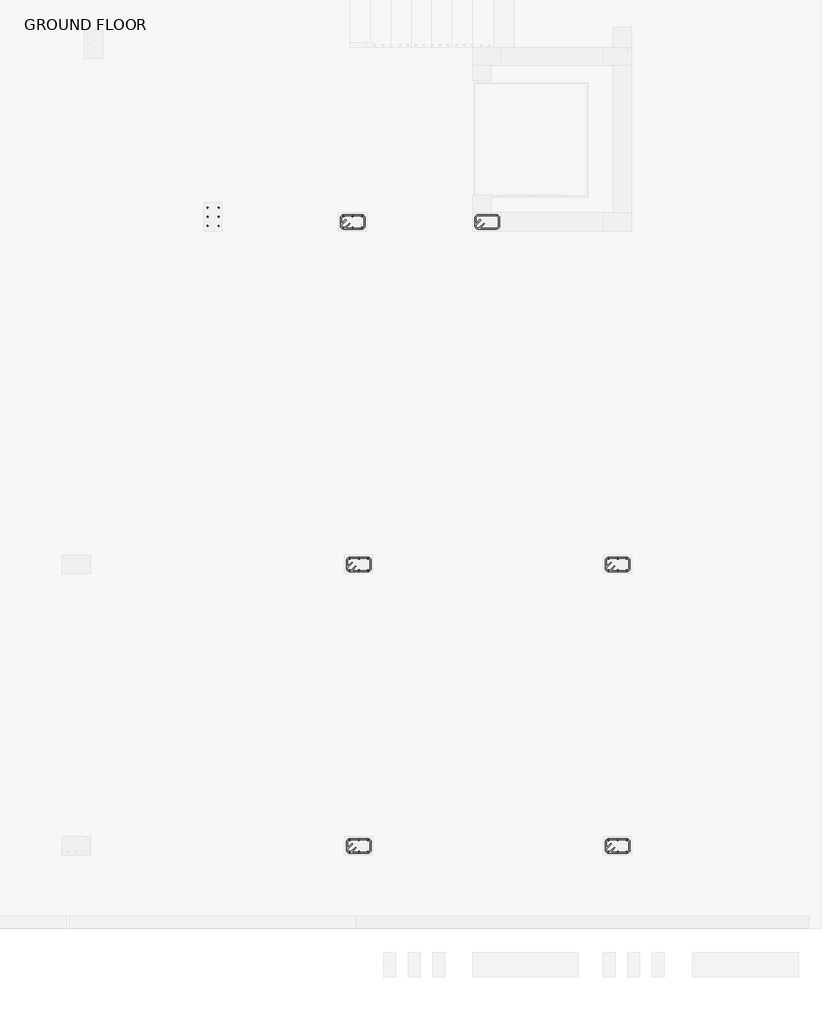
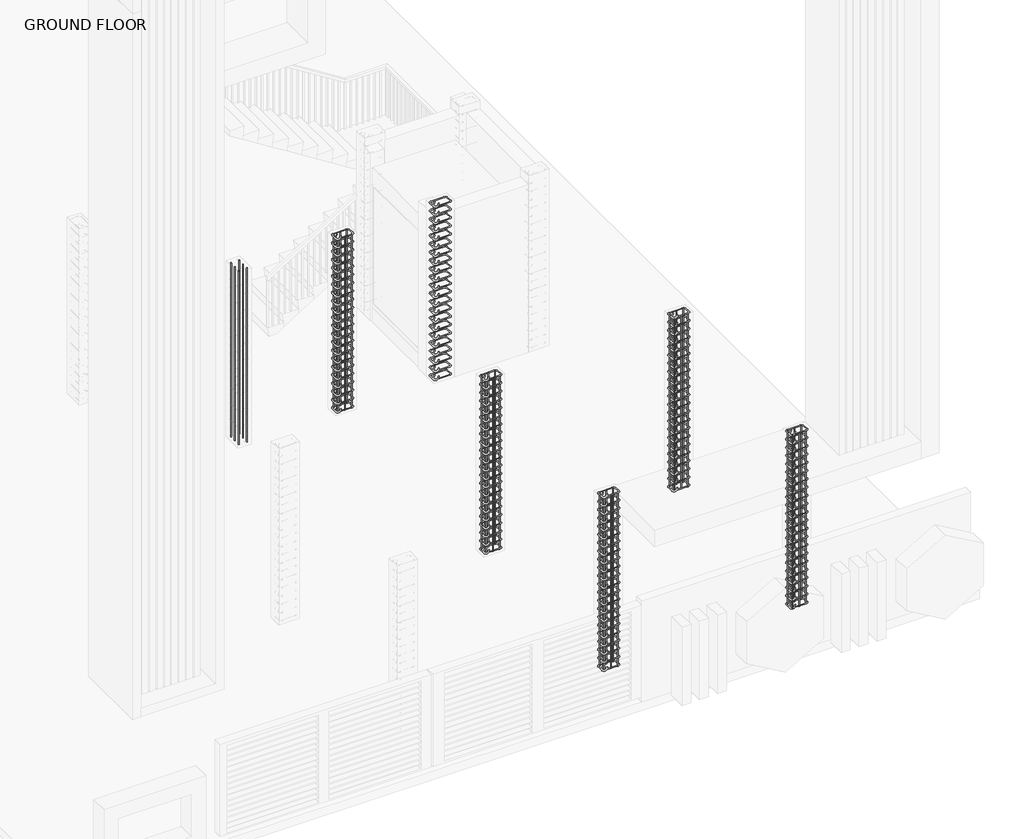
# One storey, part 4 of 7: 18 reinforcing bars.
"""IFC4 building model written with IfcOpenShell, lengths in millimetres."""

from ifc_helpers import new_model, si_unit, point, frame, origin, place, context, project, spatial, polyline, circle_curve, trimmed, segment, composite_curve, source, transform, mapped, element, save
from ifc_brep_helpers import swept_disk

model = new_model("IFC4")

# Units and contexts
model_context = context("Model", 3, world=origin())
ifc_project = project(units=[si_unit("LENGTHUNIT", "METRE", prefix="MILLI")], contexts=[model_context])

# Site, building, storey
site = spatial("IfcSite", under=ifc_project)
building = spatial("IfcBuilding", under=site)
storey = spatial("IfcBuildingStorey", under=building, Name="GROUND FLOOR", Elevation=0.0)

# Reinforcing bars
placement = place(None, origin())
reinforcing_bar_shape = source(origin(), model_context, "Body", "SolidModel", [
    swept_disk(composite_curve([segment(polyline([(2917.3487983, -2181.6091695, 3168.65), (2863.4672616, -2235.4907063, 3168.65)]), True, "CONTINUOUS"), segment(trimmed(circle_curve(frame((2841.0166213, -2213.040066, 3168.65), z_axis=(0.0, 0.0, -1.0), x_axis=(22.450640299999577, -22.450640300000032, 0.0)), 31.75), [point((2863.4672616, -2235.4907063, 3168.65))], [point((2809.2666213, -2213.040066, 3168.65))], True, "CARTESIAN"), True, "CONTINUOUS"), segment(polyline([(2809.2666213, -2213.040066, 3168.65), (2809.2666213, -2111.440066, 3168.65)]), True, "CONTINUOUS"), segment(trimmed(circle_curve(frame((2841.0166213, -2111.440066, 3168.65), z_axis=(0.0, 0.0, -1.0), x_axis=(-31.75, 0.0, 0.0)), 31.75), [point((2809.2666213, -2111.440066, 3168.65))], [point((2841.0166213, -2079.690066, 3168.65))], True, "CARTESIAN"), True, "CONTINUOUS"), segment(polyline([(2841.0166213, -2079.690066, 3168.65), (3069.6166213, -2079.690066, 3168.65)]), True, "CONTINUOUS"), segment(trimmed(circle_curve(frame((3069.6166213, -2111.3465459, 3171.0851138), z_axis=(0.0, -0.07669649888473773, -0.9970544855015816), x_axis=(0.0, 31.656479899999795, -2.4351137999997263)), 31.75), [point((3069.6166213, -2079.690066, 3168.65))], [point((3101.3666213, -2111.3465459, 3171.0851138))], True, "CARTESIAN"), True, "CONTINUOUS"), segment(polyline([(3101.3666213, -2111.3465459, 3171.0851138), (3101.3666213, -2213.1335861, 3178.9148862)]), True, "CONTINUOUS"), segment(trimmed(circle_curve(frame((3069.6166213, -2213.1335861, 3178.9148862), z_axis=(0.0, -0.07669649888473773, -0.9970544855015816), x_axis=(31.75, 0.0, 0.0)), 31.75), [point((3101.3666213, -2213.1335861, 3178.9148862))], [point((3069.6166213, -2244.790066, 3181.35))], True, "CARTESIAN"), True, "CONTINUOUS"), segment(polyline([(3069.6166213, -2244.790066, 3181.35), (2841.0166213, -2244.790066, 3181.35)]), True, "CONTINUOUS"), segment(trimmed(circle_curve(frame((2841.0166213, -2213.040066, 3181.35), z_axis=(0.0, 0.0, -1.0), x_axis=(0.0, -31.75, 0.0)), 31.75), [point((2841.0166213, -2244.790066, 3181.35))], [point((2818.565981, -2190.5894257, 3181.35))], True, "CARTESIAN"), True, "CONTINUOUS"), segment(polyline([(2818.565981, -2190.5894257, 3181.35), (2872.4475177, -2136.7078889, 3181.35)]), True, "CONTINUOUS")], self_intersect=False), 6.35),
])
element("IfcReinforcingBar", 1, at=placement, inside=storey, context=model_context, shape_type="MappedRepresentation", body=[
    mapped(reinforcing_bar_shape, transform((0.0, 0.0, 0.0), x_axis=(1.0, 0.0, 0.0), y_axis=(0.0, 1.0, 0.0), z_axis=(0.0, 0.0, 1.0))),
    mapped(reinforcing_bar_shape, transform((0.0, 0.0, -149.3761905), x_axis=(1.0, 0.0, 0.0), y_axis=(0.0, 1.0, 0.0), z_axis=(0.0, 0.0, 1.0))),
    mapped(reinforcing_bar_shape, transform((0.0, 0.0, -298.752381), x_axis=(1.0, 0.0, 0.0), y_axis=(0.0, 1.0, 0.0), z_axis=(0.0, 0.0, 1.0))),
    mapped(reinforcing_bar_shape, transform((0.0, 0.0, -448.1285714), x_axis=(1.0, 0.0, 0.0), y_axis=(0.0, 1.0, 0.0), z_axis=(0.0, 0.0, 1.0))),
    mapped(reinforcing_bar_shape, transform((0.0, 0.0, -597.5047619), x_axis=(1.0, 0.0, 0.0), y_axis=(0.0, 1.0, 0.0), z_axis=(0.0, 0.0, 1.0))),
    mapped(reinforcing_bar_shape, transform((0.0, 0.0, -746.8809524), x_axis=(1.0, 0.0, 0.0), y_axis=(0.0, 1.0, 0.0), z_axis=(0.0, 0.0, 1.0))),
    mapped(reinforcing_bar_shape, transform((0.0, 0.0, -896.2571429), x_axis=(1.0, 0.0, 0.0), y_axis=(0.0, 1.0, 0.0), z_axis=(0.0, 0.0, 1.0))),
    mapped(reinforcing_bar_shape, transform((0.0, 0.0, -1045.6333333), x_axis=(1.0, 0.0, 0.0), y_axis=(0.0, 1.0, 0.0), z_axis=(0.0, 0.0, 1.0))),
    mapped(reinforcing_bar_shape, transform((0.0, 0.0, -1195.0095238), x_axis=(1.0, 0.0, 0.0), y_axis=(0.0, 1.0, 0.0), z_axis=(0.0, 0.0, 1.0))),
    mapped(reinforcing_bar_shape, transform((0.0, 0.0, -1344.3857143), x_axis=(1.0, 0.0, 0.0), y_axis=(0.0, 1.0, 0.0), z_axis=(0.0, 0.0, 1.0))),
    mapped(reinforcing_bar_shape, transform((0.0, 0.0, -1493.7619048), x_axis=(1.0, 0.0, 0.0), y_axis=(0.0, 1.0, 0.0), z_axis=(0.0, 0.0, 1.0))),
    mapped(reinforcing_bar_shape, transform((0.0, 0.0, -1643.1380952), x_axis=(1.0, 0.0, 0.0), y_axis=(0.0, 1.0, 0.0), z_axis=(0.0, 0.0, 1.0))),
    mapped(reinforcing_bar_shape, transform((0.0, 0.0, -1792.5142857), x_axis=(1.0, 0.0, 0.0), y_axis=(0.0, 1.0, 0.0), z_axis=(0.0, 0.0, 1.0))),
    mapped(reinforcing_bar_shape, transform((0.0, 0.0, -1941.8904762), x_axis=(1.0, 0.0, 0.0), y_axis=(0.0, 1.0, 0.0), z_axis=(0.0, 0.0, 1.0))),
    mapped(reinforcing_bar_shape, transform((0.0, 0.0, -2091.2666667), x_axis=(1.0, 0.0, 0.0), y_axis=(0.0, 1.0, 0.0), z_axis=(0.0, 0.0, 1.0))),
    mapped(reinforcing_bar_shape, transform((0.0, 0.0, -2240.6428571), x_axis=(1.0, 0.0, 0.0), y_axis=(0.0, 1.0, 0.0), z_axis=(0.0, 0.0, 1.0))),
    mapped(reinforcing_bar_shape, transform((0.0, 0.0, -2390.0190476), x_axis=(1.0, 0.0, 0.0), y_axis=(0.0, 1.0, 0.0), z_axis=(0.0, 0.0, 1.0))),
    mapped(reinforcing_bar_shape, transform((0.0, 0.0, -2539.3952381), x_axis=(1.0, 0.0, 0.0), y_axis=(0.0, 1.0, 0.0), z_axis=(0.0, 0.0, 1.0))),
    mapped(reinforcing_bar_shape, transform((0.0, 0.0, -2688.7714286), x_axis=(1.0, 0.0, 0.0), y_axis=(0.0, 1.0, 0.0), z_axis=(0.0, 0.0, 1.0))),
    mapped(reinforcing_bar_shape, transform((0.0, 0.0, -2838.147619), x_axis=(1.0, 0.0, 0.0), y_axis=(0.0, 1.0, 0.0), z_axis=(0.0, 0.0, 1.0))),
    mapped(reinforcing_bar_shape, transform((0.0, 0.0, -2987.5238095), x_axis=(1.0, 0.0, 0.0), y_axis=(0.0, 1.0, 0.0), z_axis=(0.0, 0.0, 1.0))),
    mapped(reinforcing_bar_shape, transform((0.0, 0.0, -3136.9), x_axis=(1.0, 0.0, 0.0), y_axis=(0.0, 1.0, 0.0), z_axis=(0.0, 0.0, 1.0))),
])
reinforcing_bar_2_shape = source(origin(), model_context, "Body", "SolidModel", [
    swept_disk(composite_curve([segment(polyline([(1240.9487983, -2181.6091695, 3168.65), (1187.0672616, -2235.4907063, 3168.65)]), True, "CONTINUOUS"), segment(trimmed(circle_curve(frame((1164.6166213, -2213.040066, 3168.65), z_axis=(0.0, 0.0, -1.0), x_axis=(22.450640300000032, -22.450640300000032, 0.0)), 31.75), [point((1187.0672616, -2235.4907063, 3168.65))], [point((1132.8666213, -2213.040066, 3168.65))], True, "CARTESIAN"), True, "CONTINUOUS"), segment(polyline([(1132.8666213, -2213.040066, 3168.65), (1132.8666213, -2111.440066, 3168.65)]), True, "CONTINUOUS"), segment(trimmed(circle_curve(frame((1164.6166213, -2111.440066, 3168.65), z_axis=(0.0, 0.0, -1.0), x_axis=(-31.75, 0.0, 0.0)), 31.75), [point((1132.8666213, -2111.440066, 3168.65))], [point((1164.6166213, -2079.690066, 3168.65))], True, "CARTESIAN"), True, "CONTINUOUS"), segment(polyline([(1164.6166213, -2079.690066, 3168.65), (1393.2166213, -2079.690066, 3168.65)]), True, "CONTINUOUS"), segment(trimmed(circle_curve(frame((1393.2166213, -2111.3465459, 3171.0851138), z_axis=(0.0, -0.07669649888473773, -0.9970544855015816), x_axis=(0.0, 31.656479899999795, -2.4351137999997263)), 31.75), [point((1393.2166213, -2079.690066, 3168.65))], [point((1424.9666213, -2111.3465459, 3171.0851138))], True, "CARTESIAN"), True, "CONTINUOUS"), segment(polyline([(1424.9666213, -2111.3465459, 3171.0851138), (1424.9666213, -2213.1335861, 3178.9148862)]), True, "CONTINUOUS"), segment(trimmed(circle_curve(frame((1393.2166213, -2213.1335861, 3178.9148862), z_axis=(0.0, -0.07669649888473773, -0.9970544855015816), x_axis=(31.75, 0.0, 0.0)), 31.75), [point((1424.9666213, -2213.1335861, 3178.9148862))], [point((1393.2166213, -2244.790066, 3181.35))], True, "CARTESIAN"), True, "CONTINUOUS"), segment(polyline([(1393.2166213, -2244.790066, 3181.35), (1164.6166213, -2244.790066, 3181.35)]), True, "CONTINUOUS"), segment(trimmed(circle_curve(frame((1164.6166213, -2213.040066, 3181.35), z_axis=(0.0, 0.0, -1.0), x_axis=(0.0, -31.75, 0.0)), 31.75), [point((1164.6166213, -2244.790066, 3181.35))], [point((1142.165981, -2190.5894257, 3181.35))], True, "CARTESIAN"), True, "CONTINUOUS"), segment(polyline([(1142.165981, -2190.5894257, 3181.35), (1196.0475177, -2136.7078889, 3181.35)]), True, "CONTINUOUS")], self_intersect=False), 6.35),
])
element("IfcReinforcingBar", 2, at=placement, inside=storey, context=model_context, shape_type="MappedRepresentation", body=[
    mapped(reinforcing_bar_2_shape, transform((0.0, 0.0, 0.0), x_axis=(1.0, 0.0, 0.0), y_axis=(0.0, 1.0, 0.0), z_axis=(0.0, 0.0, 1.0))),
    mapped(reinforcing_bar_2_shape, transform((0.0, 0.0, -149.3761905), x_axis=(1.0, 0.0, 0.0), y_axis=(0.0, 1.0, 0.0), z_axis=(0.0, 0.0, 1.0))),
    mapped(reinforcing_bar_2_shape, transform((0.0, 0.0, -298.752381), x_axis=(1.0, 0.0, 0.0), y_axis=(0.0, 1.0, 0.0), z_axis=(0.0, 0.0, 1.0))),
    mapped(reinforcing_bar_2_shape, transform((0.0, 0.0, -448.1285714), x_axis=(1.0, 0.0, 0.0), y_axis=(0.0, 1.0, 0.0), z_axis=(0.0, 0.0, 1.0))),
    mapped(reinforcing_bar_2_shape, transform((0.0, 0.0, -597.5047619), x_axis=(1.0, 0.0, 0.0), y_axis=(0.0, 1.0, 0.0), z_axis=(0.0, 0.0, 1.0))),
    mapped(reinforcing_bar_2_shape, transform((0.0, 0.0, -746.8809524), x_axis=(1.0, 0.0, 0.0), y_axis=(0.0, 1.0, 0.0), z_axis=(0.0, 0.0, 1.0))),
    mapped(reinforcing_bar_2_shape, transform((0.0, 0.0, -896.2571429), x_axis=(1.0, 0.0, 0.0), y_axis=(0.0, 1.0, 0.0), z_axis=(0.0, 0.0, 1.0))),
    mapped(reinforcing_bar_2_shape, transform((0.0, 0.0, -1045.6333333), x_axis=(1.0, 0.0, 0.0), y_axis=(0.0, 1.0, 0.0), z_axis=(0.0, 0.0, 1.0))),
    mapped(reinforcing_bar_2_shape, transform((0.0, 0.0, -1195.0095238), x_axis=(1.0, 0.0, 0.0), y_axis=(0.0, 1.0, 0.0), z_axis=(0.0, 0.0, 1.0))),
    mapped(reinforcing_bar_2_shape, transform((0.0, 0.0, -1344.3857143), x_axis=(1.0, 0.0, 0.0), y_axis=(0.0, 1.0, 0.0), z_axis=(0.0, 0.0, 1.0))),
    mapped(reinforcing_bar_2_shape, transform((0.0, 0.0, -1493.7619048), x_axis=(1.0, 0.0, 0.0), y_axis=(0.0, 1.0, 0.0), z_axis=(0.0, 0.0, 1.0))),
    mapped(reinforcing_bar_2_shape, transform((0.0, 0.0, -1643.1380952), x_axis=(1.0, 0.0, 0.0), y_axis=(0.0, 1.0, 0.0), z_axis=(0.0, 0.0, 1.0))),
    mapped(reinforcing_bar_2_shape, transform((0.0, 0.0, -1792.5142857), x_axis=(1.0, 0.0, 0.0), y_axis=(0.0, 1.0, 0.0), z_axis=(0.0, 0.0, 1.0))),
    mapped(reinforcing_bar_2_shape, transform((0.0, 0.0, -1941.8904762), x_axis=(1.0, 0.0, 0.0), y_axis=(0.0, 1.0, 0.0), z_axis=(0.0, 0.0, 1.0))),
    mapped(reinforcing_bar_2_shape, transform((0.0, 0.0, -2091.2666667), x_axis=(1.0, 0.0, 0.0), y_axis=(0.0, 1.0, 0.0), z_axis=(0.0, 0.0, 1.0))),
    mapped(reinforcing_bar_2_shape, transform((0.0, 0.0, -2240.6428571), x_axis=(1.0, 0.0, 0.0), y_axis=(0.0, 1.0, 0.0), z_axis=(0.0, 0.0, 1.0))),
    mapped(reinforcing_bar_2_shape, transform((0.0, 0.0, -2390.0190476), x_axis=(1.0, 0.0, 0.0), y_axis=(0.0, 1.0, 0.0), z_axis=(0.0, 0.0, 1.0))),
    mapped(reinforcing_bar_2_shape, transform((0.0, 0.0, -2539.3952381), x_axis=(1.0, 0.0, 0.0), y_axis=(0.0, 1.0, 0.0), z_axis=(0.0, 0.0, 1.0))),
    mapped(reinforcing_bar_2_shape, transform((0.0, 0.0, -2688.7714286), x_axis=(1.0, 0.0, 0.0), y_axis=(0.0, 1.0, 0.0), z_axis=(0.0, 0.0, 1.0))),
    mapped(reinforcing_bar_2_shape, transform((0.0, 0.0, -2838.147619), x_axis=(1.0, 0.0, 0.0), y_axis=(0.0, 1.0, 0.0), z_axis=(0.0, 0.0, 1.0))),
    mapped(reinforcing_bar_2_shape, transform((0.0, 0.0, -2987.5238095), x_axis=(1.0, 0.0, 0.0), y_axis=(0.0, 1.0, 0.0), z_axis=(0.0, 0.0, 1.0))),
    mapped(reinforcing_bar_2_shape, transform((0.0, 0.0, -3136.9), x_axis=(1.0, 0.0, 0.0), y_axis=(0.0, 1.0, 0.0), z_axis=(0.0, 0.0, 1.0))),
])
reinforcing_bar_3_shape = source(origin(), model_context, "Body", "SolidModel", [
    swept_disk(composite_curve([segment(polyline([(1164.6166213, -2092.390066, 3175.0), (1164.6166213, -2092.390066, 25.4)]), True, "CONTINUOUS")], self_intersect=False), 6.35),
])
element("IfcReinforcingBar", 3, at=placement, inside=storey, context=model_context, shape_type="MappedRepresentation", body=[
    mapped(reinforcing_bar_3_shape, transform((0.0, 0.0, 0.0), x_axis=(1.0, 0.0, 0.0), y_axis=(0.0, 1.0, 0.0), z_axis=(0.0, 0.0, 1.0))),
    mapped(reinforcing_bar_3_shape, transform((114.3, 0.0, 0.0), x_axis=(1.0, 0.0, 0.0), y_axis=(0.0, 1.0, 0.0), z_axis=(0.0, 0.0, 1.0))),
    mapped(reinforcing_bar_3_shape, transform((228.6, 0.0, 0.0), x_axis=(1.0, 0.0, 0.0), y_axis=(0.0, 1.0, 0.0), z_axis=(0.0, 0.0, 1.0))),
])
reinforcing_bar_4_shape = source(origin(), model_context, "Body", "SolidModel", [
    swept_disk(composite_curve([segment(polyline([(1164.6166213, -2232.090066, 25.4), (1164.6166213, -2232.090066, 3175.0)]), True, "CONTINUOUS")], self_intersect=False), 6.35),
])
element("IfcReinforcingBar", 4, at=placement, inside=storey, context=model_context, shape_type="MappedRepresentation", body=[
    mapped(reinforcing_bar_4_shape, transform((0.0, 0.0, 0.0), x_axis=(1.0, 0.0, 0.0), y_axis=(0.0, 1.0, 0.0), z_axis=(0.0, 0.0, 1.0))),
    mapped(reinforcing_bar_4_shape, transform((114.3, 0.0, 0.0), x_axis=(1.0, 0.0, 0.0), y_axis=(0.0, 1.0, 0.0), z_axis=(0.0, 0.0, 1.0))),
    mapped(reinforcing_bar_4_shape, transform((228.6, 0.0, 0.0), x_axis=(1.0, 0.0, 0.0), y_axis=(0.0, 1.0, 0.0), z_axis=(0.0, 0.0, 1.0))),
])
reinforcing_bar_5_shape = source(origin(), model_context, "Body", "SolidModel", [
    swept_disk(composite_curve([segment(polyline([(-530.8333787, -2213.040066, 3175.0), (-530.8333787, -2213.040066, 25.4)]), True, "CONTINUOUS")], self_intersect=False), 6.35),
])
element("IfcReinforcingBar", 5, at=placement, inside=storey, context=model_context, shape_type="MappedRepresentation", body=[
    mapped(reinforcing_bar_5_shape, transform((0.0, 0.0, 0.0), x_axis=(1.0, 0.0, 0.0), y_axis=(0.0, 1.0, 0.0), z_axis=(0.0, 0.0, 1.0))),
    mapped(reinforcing_bar_5_shape, transform((0.0, 114.3, 0.0), x_axis=(1.0, 0.0, 0.0), y_axis=(0.0, 1.0, 0.0), z_axis=(0.0, 0.0, 1.0))),
    mapped(reinforcing_bar_5_shape, transform((0.0, 228.6, 0.0), x_axis=(1.0, 0.0, 0.0), y_axis=(0.0, 1.0, 0.0), z_axis=(0.0, 0.0, 1.0))),
])
reinforcing_bar_6_shape = source(origin(), model_context, "Body", "SolidModel", [
    swept_disk(composite_curve([segment(polyline([(-391.1333787, -2213.040066, 25.4), (-391.1333787, -2213.040066, 3175.0)]), True, "CONTINUOUS")], self_intersect=False), 6.35),
])
element("IfcReinforcingBar", 6, at=placement, inside=storey, context=model_context, shape_type="MappedRepresentation", body=[
    mapped(reinforcing_bar_6_shape, transform((0.0, 0.0, 0.0), x_axis=(1.0, 0.0, 0.0), y_axis=(0.0, 1.0, 0.0), z_axis=(0.0, 0.0, 1.0))),
    mapped(reinforcing_bar_6_shape, transform((0.0, 114.3, 0.0), x_axis=(1.0, 0.0, 0.0), y_axis=(0.0, 1.0, 0.0), z_axis=(0.0, 0.0, 1.0))),
    mapped(reinforcing_bar_6_shape, transform((0.0, 228.6, 0.0), x_axis=(1.0, 0.0, 0.0), y_axis=(0.0, 1.0, 0.0), z_axis=(0.0, 0.0, 1.0))),
])
reinforcing_bar_7_shape = source(origin(), model_context, "Body", "SolidModel", [
    swept_disk(composite_curve([segment(polyline([(4542.9487983, -6448.8091695, 3168.65), (4489.0672616, -6502.6907063, 3168.65)]), True, "CONTINUOUS"), segment(trimmed(circle_curve(frame((4466.6166213, -6480.240066, 3168.65), z_axis=(0.0, 0.0, -1.0), x_axis=(22.450640300000487, -22.450640299999577, 0.0)), 31.75), [point((4489.0672616, -6502.6907063, 3168.65))], [point((4434.8666213, -6480.240066, 3168.65))], True, "CARTESIAN"), True, "CONTINUOUS"), segment(polyline([(4434.8666213, -6480.240066, 3168.65), (4434.8666213, -6378.640066, 3168.65)]), True, "CONTINUOUS"), segment(trimmed(circle_curve(frame((4466.6166213, -6378.640066, 3168.65), z_axis=(0.0, 0.0, -1.0), x_axis=(-31.75, 0.0, 0.0)), 31.75), [point((4434.8666213, -6378.640066, 3168.65))], [point((4466.6166213, -6346.890066, 3168.65))], True, "CARTESIAN"), True, "CONTINUOUS"), segment(polyline([(4466.6166213, -6346.890066, 3168.65), (4695.2166213, -6346.890066, 3168.65)]), True, "CONTINUOUS"), segment(trimmed(circle_curve(frame((4695.2166213, -6378.5465459, 3171.0851138), z_axis=(0.0, -0.07669649888473773, -0.9970544855015816), x_axis=(0.0, 31.656479899999795, -2.4351137999997263)), 31.75), [point((4695.2166213, -6346.890066, 3168.65))], [point((4726.9666213, -6378.5465459, 3171.0851138))], True, "CARTESIAN"), True, "CONTINUOUS"), segment(polyline([(4726.9666213, -6378.5465459, 3171.0851138), (4726.9666213, -6480.3335861, 3178.9148862)]), True, "CONTINUOUS"), segment(trimmed(circle_curve(frame((4695.2166213, -6480.3335861, 3178.9148862), z_axis=(0.0, -0.07669649888473773, -0.9970544855015816), x_axis=(31.75, 0.0, 0.0)), 31.75), [point((4726.9666213, -6480.3335861, 3178.9148862))], [point((4695.2166213, -6511.990066, 3181.35))], True, "CARTESIAN"), True, "CONTINUOUS"), segment(polyline([(4695.2166213, -6511.990066, 3181.35), (4466.6166213, -6511.990066, 3181.35)]), True, "CONTINUOUS"), segment(trimmed(circle_curve(frame((4466.6166213, -6480.240066, 3181.35), z_axis=(0.0, 0.0, -1.0), x_axis=(0.0, -31.75, 0.0)), 31.75), [point((4466.6166213, -6511.990066, 3181.35))], [point((4444.165981, -6457.7894257, 3181.35))], True, "CARTESIAN"), True, "CONTINUOUS"), segment(polyline([(4444.165981, -6457.7894257, 3181.35), (4498.0475177, -6403.9078889, 3181.35)]), True, "CONTINUOUS")], self_intersect=False), 6.35),
])
element("IfcReinforcingBar", 7, at=placement, inside=storey, context=model_context, shape_type="MappedRepresentation", body=[
    mapped(reinforcing_bar_7_shape, transform((0.0, 0.0, 0.0), x_axis=(1.0, 0.0, 0.0), y_axis=(0.0, 1.0, 0.0), z_axis=(0.0, 0.0, 1.0))),
    mapped(reinforcing_bar_7_shape, transform((0.0, 0.0, -149.3761905), x_axis=(1.0, 0.0, 0.0), y_axis=(0.0, 1.0, 0.0), z_axis=(0.0, 0.0, 1.0))),
    mapped(reinforcing_bar_7_shape, transform((0.0, 0.0, -298.752381), x_axis=(1.0, 0.0, 0.0), y_axis=(0.0, 1.0, 0.0), z_axis=(0.0, 0.0, 1.0))),
    mapped(reinforcing_bar_7_shape, transform((0.0, 0.0, -448.1285714), x_axis=(1.0, 0.0, 0.0), y_axis=(0.0, 1.0, 0.0), z_axis=(0.0, 0.0, 1.0))),
    mapped(reinforcing_bar_7_shape, transform((0.0, 0.0, -597.5047619), x_axis=(1.0, 0.0, 0.0), y_axis=(0.0, 1.0, 0.0), z_axis=(0.0, 0.0, 1.0))),
    mapped(reinforcing_bar_7_shape, transform((0.0, 0.0, -746.8809524), x_axis=(1.0, 0.0, 0.0), y_axis=(0.0, 1.0, 0.0), z_axis=(0.0, 0.0, 1.0))),
    mapped(reinforcing_bar_7_shape, transform((0.0, 0.0, -896.2571429), x_axis=(1.0, 0.0, 0.0), y_axis=(0.0, 1.0, 0.0), z_axis=(0.0, 0.0, 1.0))),
    mapped(reinforcing_bar_7_shape, transform((0.0, 0.0, -1045.6333333), x_axis=(1.0, 0.0, 0.0), y_axis=(0.0, 1.0, 0.0), z_axis=(0.0, 0.0, 1.0))),
    mapped(reinforcing_bar_7_shape, transform((0.0, 0.0, -1195.0095238), x_axis=(1.0, 0.0, 0.0), y_axis=(0.0, 1.0, 0.0), z_axis=(0.0, 0.0, 1.0))),
    mapped(reinforcing_bar_7_shape, transform((0.0, 0.0, -1344.3857143), x_axis=(1.0, 0.0, 0.0), y_axis=(0.0, 1.0, 0.0), z_axis=(0.0, 0.0, 1.0))),
    mapped(reinforcing_bar_7_shape, transform((0.0, 0.0, -1493.7619048), x_axis=(1.0, 0.0, 0.0), y_axis=(0.0, 1.0, 0.0), z_axis=(0.0, 0.0, 1.0))),
    mapped(reinforcing_bar_7_shape, transform((0.0, 0.0, -1643.1380952), x_axis=(1.0, 0.0, 0.0), y_axis=(0.0, 1.0, 0.0), z_axis=(0.0, 0.0, 1.0))),
    mapped(reinforcing_bar_7_shape, transform((0.0, 0.0, -1792.5142857), x_axis=(1.0, 0.0, 0.0), y_axis=(0.0, 1.0, 0.0), z_axis=(0.0, 0.0, 1.0))),
    mapped(reinforcing_bar_7_shape, transform((0.0, 0.0, -1941.8904762), x_axis=(1.0, 0.0, 0.0), y_axis=(0.0, 1.0, 0.0), z_axis=(0.0, 0.0, 1.0))),
    mapped(reinforcing_bar_7_shape, transform((0.0, 0.0, -2091.2666667), x_axis=(1.0, 0.0, 0.0), y_axis=(0.0, 1.0, 0.0), z_axis=(0.0, 0.0, 1.0))),
    mapped(reinforcing_bar_7_shape, transform((0.0, 0.0, -2240.6428571), x_axis=(1.0, 0.0, 0.0), y_axis=(0.0, 1.0, 0.0), z_axis=(0.0, 0.0, 1.0))),
    mapped(reinforcing_bar_7_shape, transform((0.0, 0.0, -2390.0190476), x_axis=(1.0, 0.0, 0.0), y_axis=(0.0, 1.0, 0.0), z_axis=(0.0, 0.0, 1.0))),
    mapped(reinforcing_bar_7_shape, transform((0.0, 0.0, -2539.3952381), x_axis=(1.0, 0.0, 0.0), y_axis=(0.0, 1.0, 0.0), z_axis=(0.0, 0.0, 1.0))),
    mapped(reinforcing_bar_7_shape, transform((0.0, 0.0, -2688.7714286), x_axis=(1.0, 0.0, 0.0), y_axis=(0.0, 1.0, 0.0), z_axis=(0.0, 0.0, 1.0))),
    mapped(reinforcing_bar_7_shape, transform((0.0, 0.0, -2838.147619), x_axis=(1.0, 0.0, 0.0), y_axis=(0.0, 1.0, 0.0), z_axis=(0.0, 0.0, 1.0))),
    mapped(reinforcing_bar_7_shape, transform((0.0, 0.0, -2987.5238095), x_axis=(1.0, 0.0, 0.0), y_axis=(0.0, 1.0, 0.0), z_axis=(0.0, 0.0, 1.0))),
    mapped(reinforcing_bar_7_shape, transform((0.0, 0.0, -3136.9), x_axis=(1.0, 0.0, 0.0), y_axis=(0.0, 1.0, 0.0), z_axis=(0.0, 0.0, 1.0))),
])
reinforcing_bar_8_shape = source(origin(), model_context, "Body", "SolidModel", [
    swept_disk(composite_curve([segment(polyline([(4466.6166213, -6359.590066, 3175.0), (4466.6166213, -6359.590066, 25.4)]), True, "CONTINUOUS")], self_intersect=False), 6.35),
])
element("IfcReinforcingBar", 8, at=placement, inside=storey, context=model_context, shape_type="MappedRepresentation", body=[
    mapped(reinforcing_bar_8_shape, transform((0.0, 0.0, 0.0), x_axis=(1.0, 0.0, 0.0), y_axis=(0.0, 1.0, 0.0), z_axis=(0.0, 0.0, 1.0))),
    mapped(reinforcing_bar_8_shape, transform((114.3, 0.0, 0.0), x_axis=(1.0, 0.0, 0.0), y_axis=(0.0, 1.0, 0.0), z_axis=(0.0, 0.0, 1.0))),
    mapped(reinforcing_bar_8_shape, transform((228.6, 0.0, 0.0), x_axis=(1.0, 0.0, 0.0), y_axis=(0.0, 1.0, 0.0), z_axis=(0.0, 0.0, 1.0))),
])
reinforcing_bar_9_shape = source(origin(), model_context, "Body", "SolidModel", [
    swept_disk(composite_curve([segment(polyline([(4466.6166213, -6499.290066, 25.4), (4466.6166213, -6499.290066, 3175.0)]), True, "CONTINUOUS")], self_intersect=False), 6.35),
])
element("IfcReinforcingBar", 9, at=placement, inside=storey, context=model_context, shape_type="MappedRepresentation", body=[
    mapped(reinforcing_bar_9_shape, transform((0.0, 0.0, 0.0), x_axis=(1.0, 0.0, 0.0), y_axis=(0.0, 1.0, 0.0), z_axis=(0.0, 0.0, 1.0))),
    mapped(reinforcing_bar_9_shape, transform((114.3, 0.0, 0.0), x_axis=(1.0, 0.0, 0.0), y_axis=(0.0, 1.0, 0.0), z_axis=(0.0, 0.0, 1.0))),
    mapped(reinforcing_bar_9_shape, transform((228.6, 0.0, 0.0), x_axis=(1.0, 0.0, 0.0), y_axis=(0.0, 1.0, 0.0), z_axis=(0.0, 0.0, 1.0))),
])
reinforcing_bar_10_shape = source(origin(), model_context, "Body", "SolidModel", [
    swept_disk(composite_curve([segment(polyline([(1317.1487983, -6448.8091695, 3168.65), (1263.2672616, -6502.6907063, 3168.65)]), True, "CONTINUOUS"), segment(trimmed(circle_curve(frame((1240.8166213, -6480.240066, 3168.65), z_axis=(0.0, 0.0, -1.0), x_axis=(22.450640300000032, -22.450640299999577, 0.0)), 31.75), [point((1263.2672616, -6502.6907063, 3168.65))], [point((1209.0666213, -6480.240066, 3168.65))], True, "CARTESIAN"), True, "CONTINUOUS"), segment(polyline([(1209.0666213, -6480.240066, 3168.65), (1209.0666213, -6378.640066, 3168.65)]), True, "CONTINUOUS"), segment(trimmed(circle_curve(frame((1240.8166213, -6378.640066, 3168.65), z_axis=(0.0, 0.0, -1.0), x_axis=(-31.75, 0.0, 0.0)), 31.75), [point((1209.0666213, -6378.640066, 3168.65))], [point((1240.8166213, -6346.890066, 3168.65))], True, "CARTESIAN"), True, "CONTINUOUS"), segment(polyline([(1240.8166213, -6346.890066, 3168.65), (1469.4166213, -6346.890066, 3168.65)]), True, "CONTINUOUS"), segment(trimmed(circle_curve(frame((1469.4166213, -6378.5465459, 3171.0851138), z_axis=(0.0, -0.07669649888473773, -0.9970544855015816), x_axis=(0.0, 31.656479899999795, -2.4351137999997263)), 31.75), [point((1469.4166213, -6346.890066, 3168.65))], [point((1501.1666213, -6378.5465459, 3171.0851138))], True, "CARTESIAN"), True, "CONTINUOUS"), segment(polyline([(1501.1666213, -6378.5465459, 3171.0851138), (1501.1666213, -6480.3335861, 3178.9148862)]), True, "CONTINUOUS"), segment(trimmed(circle_curve(frame((1469.4166213, -6480.3335861, 3178.9148862), z_axis=(0.0, -0.07669649888473773, -0.9970544855015816), x_axis=(31.75, 0.0, 0.0)), 31.75), [point((1501.1666213, -6480.3335861, 3178.9148862))], [point((1469.4166213, -6511.990066, 3181.35))], True, "CARTESIAN"), True, "CONTINUOUS"), segment(polyline([(1469.4166213, -6511.990066, 3181.35), (1240.8166213, -6511.990066, 3181.35)]), True, "CONTINUOUS"), segment(trimmed(circle_curve(frame((1240.8166213, -6480.240066, 3181.35), z_axis=(0.0, 0.0, -1.0), x_axis=(0.0, -31.75, 0.0)), 31.75), [point((1240.8166213, -6511.990066, 3181.35))], [point((1218.365981, -6457.7894257, 3181.35))], True, "CARTESIAN"), True, "CONTINUOUS"), segment(polyline([(1218.365981, -6457.7894257, 3181.35), (1272.2475177, -6403.9078889, 3181.35)]), True, "CONTINUOUS")], self_intersect=False), 6.35),
])
element("IfcReinforcingBar", 10, at=placement, inside=storey, context=model_context, shape_type="MappedRepresentation", body=[
    mapped(reinforcing_bar_10_shape, transform((0.0, 0.0, 0.0), x_axis=(1.0, 0.0, 0.0), y_axis=(0.0, 1.0, 0.0), z_axis=(0.0, 0.0, 1.0))),
    mapped(reinforcing_bar_10_shape, transform((0.0, 0.0, -149.3761905), x_axis=(1.0, 0.0, 0.0), y_axis=(0.0, 1.0, 0.0), z_axis=(0.0, 0.0, 1.0))),
    mapped(reinforcing_bar_10_shape, transform((0.0, 0.0, -298.752381), x_axis=(1.0, 0.0, 0.0), y_axis=(0.0, 1.0, 0.0), z_axis=(0.0, 0.0, 1.0))),
    mapped(reinforcing_bar_10_shape, transform((0.0, 0.0, -448.1285714), x_axis=(1.0, 0.0, 0.0), y_axis=(0.0, 1.0, 0.0), z_axis=(0.0, 0.0, 1.0))),
    mapped(reinforcing_bar_10_shape, transform((0.0, 0.0, -597.5047619), x_axis=(1.0, 0.0, 0.0), y_axis=(0.0, 1.0, 0.0), z_axis=(0.0, 0.0, 1.0))),
    mapped(reinforcing_bar_10_shape, transform((0.0, 0.0, -746.8809524), x_axis=(1.0, 0.0, 0.0), y_axis=(0.0, 1.0, 0.0), z_axis=(0.0, 0.0, 1.0))),
    mapped(reinforcing_bar_10_shape, transform((0.0, 0.0, -896.2571429), x_axis=(1.0, 0.0, 0.0), y_axis=(0.0, 1.0, 0.0), z_axis=(0.0, 0.0, 1.0))),
    mapped(reinforcing_bar_10_shape, transform((0.0, 0.0, -1045.6333333), x_axis=(1.0, 0.0, 0.0), y_axis=(0.0, 1.0, 0.0), z_axis=(0.0, 0.0, 1.0))),
    mapped(reinforcing_bar_10_shape, transform((0.0, 0.0, -1195.0095238), x_axis=(1.0, 0.0, 0.0), y_axis=(0.0, 1.0, 0.0), z_axis=(0.0, 0.0, 1.0))),
    mapped(reinforcing_bar_10_shape, transform((0.0, 0.0, -1344.3857143), x_axis=(1.0, 0.0, 0.0), y_axis=(0.0, 1.0, 0.0), z_axis=(0.0, 0.0, 1.0))),
    mapped(reinforcing_bar_10_shape, transform((0.0, 0.0, -1493.7619048), x_axis=(1.0, 0.0, 0.0), y_axis=(0.0, 1.0, 0.0), z_axis=(0.0, 0.0, 1.0))),
    mapped(reinforcing_bar_10_shape, transform((0.0, 0.0, -1643.1380952), x_axis=(1.0, 0.0, 0.0), y_axis=(0.0, 1.0, 0.0), z_axis=(0.0, 0.0, 1.0))),
    mapped(reinforcing_bar_10_shape, transform((0.0, 0.0, -1792.5142857), x_axis=(1.0, 0.0, 0.0), y_axis=(0.0, 1.0, 0.0), z_axis=(0.0, 0.0, 1.0))),
    mapped(reinforcing_bar_10_shape, transform((0.0, 0.0, -1941.8904762), x_axis=(1.0, 0.0, 0.0), y_axis=(0.0, 1.0, 0.0), z_axis=(0.0, 0.0, 1.0))),
    mapped(reinforcing_bar_10_shape, transform((0.0, 0.0, -2091.2666667), x_axis=(1.0, 0.0, 0.0), y_axis=(0.0, 1.0, 0.0), z_axis=(0.0, 0.0, 1.0))),
    mapped(reinforcing_bar_10_shape, transform((0.0, 0.0, -2240.6428571), x_axis=(1.0, 0.0, 0.0), y_axis=(0.0, 1.0, 0.0), z_axis=(0.0, 0.0, 1.0))),
    mapped(reinforcing_bar_10_shape, transform((0.0, 0.0, -2390.0190476), x_axis=(1.0, 0.0, 0.0), y_axis=(0.0, 1.0, 0.0), z_axis=(0.0, 0.0, 1.0))),
    mapped(reinforcing_bar_10_shape, transform((0.0, 0.0, -2539.3952381), x_axis=(1.0, 0.0, 0.0), y_axis=(0.0, 1.0, 0.0), z_axis=(0.0, 0.0, 1.0))),
    mapped(reinforcing_bar_10_shape, transform((0.0, 0.0, -2688.7714286), x_axis=(1.0, 0.0, 0.0), y_axis=(0.0, 1.0, 0.0), z_axis=(0.0, 0.0, 1.0))),
    mapped(reinforcing_bar_10_shape, transform((0.0, 0.0, -2838.147619), x_axis=(1.0, 0.0, 0.0), y_axis=(0.0, 1.0, 0.0), z_axis=(0.0, 0.0, 1.0))),
    mapped(reinforcing_bar_10_shape, transform((0.0, 0.0, -2987.5238095), x_axis=(1.0, 0.0, 0.0), y_axis=(0.0, 1.0, 0.0), z_axis=(0.0, 0.0, 1.0))),
    mapped(reinforcing_bar_10_shape, transform((0.0, 0.0, -3136.9), x_axis=(1.0, 0.0, 0.0), y_axis=(0.0, 1.0, 0.0), z_axis=(0.0, 0.0, 1.0))),
])
reinforcing_bar_11_shape = source(origin(), model_context, "Body", "SolidModel", [
    swept_disk(composite_curve([segment(polyline([(1240.8166213, -6359.590066, 3175.0), (1240.8166213, -6359.590066, 25.4)]), True, "CONTINUOUS")], self_intersect=False), 6.35),
])
element("IfcReinforcingBar", 11, at=placement, inside=storey, context=model_context, shape_type="MappedRepresentation", body=[
    mapped(reinforcing_bar_11_shape, transform((0.0, 0.0, 0.0), x_axis=(1.0, 0.0, 0.0), y_axis=(0.0, 1.0, 0.0), z_axis=(0.0, 0.0, 1.0))),
    mapped(reinforcing_bar_11_shape, transform((114.3, 0.0, 0.0), x_axis=(1.0, 0.0, 0.0), y_axis=(0.0, 1.0, 0.0), z_axis=(0.0, 0.0, 1.0))),
    mapped(reinforcing_bar_11_shape, transform((228.6, 0.0, 0.0), x_axis=(1.0, 0.0, 0.0), y_axis=(0.0, 1.0, 0.0), z_axis=(0.0, 0.0, 1.0))),
])
reinforcing_bar_12_shape = source(origin(), model_context, "Body", "SolidModel", [
    swept_disk(composite_curve([segment(polyline([(1240.8166213, -6499.290066, 25.4), (1240.8166213, -6499.290066, 3175.0)]), True, "CONTINUOUS")], self_intersect=False), 6.35),
])
element("IfcReinforcingBar", 12, at=placement, inside=storey, context=model_context, shape_type="MappedRepresentation", body=[
    mapped(reinforcing_bar_12_shape, transform((0.0, 0.0, 0.0), x_axis=(1.0, 0.0, 0.0), y_axis=(0.0, 1.0, 0.0), z_axis=(0.0, 0.0, 1.0))),
    mapped(reinforcing_bar_12_shape, transform((114.3, 0.0, 0.0), x_axis=(1.0, 0.0, 0.0), y_axis=(0.0, 1.0, 0.0), z_axis=(0.0, 0.0, 1.0))),
    mapped(reinforcing_bar_12_shape, transform((228.6, 0.0, 0.0), x_axis=(1.0, 0.0, 0.0), y_axis=(0.0, 1.0, 0.0), z_axis=(0.0, 0.0, 1.0))),
])
reinforcing_bar_13_shape = source(origin(), model_context, "Body", "SolidModel", [
    swept_disk(composite_curve([segment(polyline([(4542.9487983, -9954.0091695, 3168.65), (4489.0672616, -10007.8907063, 3168.65)]), True, "CONTINUOUS"), segment(trimmed(circle_curve(frame((4466.6166213, -9985.440066, 3168.65), z_axis=(0.0, 0.0, -1.0), x_axis=(22.450640300000487, -22.450640300001396, 0.0)), 31.75), [point((4489.0672616, -10007.8907063, 3168.65))], [point((4434.8666213, -9985.440066, 3168.65))], True, "CARTESIAN"), True, "CONTINUOUS"), segment(polyline([(4434.8666213, -9985.440066, 3168.65), (4434.8666213, -9883.840066, 3168.65)]), True, "CONTINUOUS"), segment(trimmed(circle_curve(frame((4466.6166213, -9883.840066, 3168.65), z_axis=(0.0, 0.0, -1.0), x_axis=(-31.75, 0.0, 0.0)), 31.75), [point((4434.8666213, -9883.840066, 3168.65))], [point((4466.6166213, -9852.090066, 3168.65))], True, "CARTESIAN"), True, "CONTINUOUS"), segment(polyline([(4466.6166213, -9852.090066, 3168.65), (4695.2166213, -9852.090066, 3168.65)]), True, "CONTINUOUS"), segment(trimmed(circle_curve(frame((4695.2166213, -9883.7465459, 3171.0851138), z_axis=(0.0, -0.07669649888473773, -0.9970544855015816), x_axis=(0.0, 31.656479899998885, -2.4351137999997263)), 31.75), [point((4695.2166213, -9852.090066, 3168.65))], [point((4726.9666213, -9883.7465459, 3171.0851138))], True, "CARTESIAN"), True, "CONTINUOUS"), segment(polyline([(4726.9666213, -9883.7465459, 3171.0851138), (4726.9666213, -9985.5335861, 3178.9148862)]), True, "CONTINUOUS"), segment(trimmed(circle_curve(frame((4695.2166213, -9985.5335861, 3178.9148862), z_axis=(0.0, -0.07669649888473773, -0.9970544855015816), x_axis=(31.75, 0.0, 0.0)), 31.75), [point((4726.9666213, -9985.5335861, 3178.9148862))], [point((4695.2166213, -10017.190066, 3181.35))], True, "CARTESIAN"), True, "CONTINUOUS"), segment(polyline([(4695.2166213, -10017.190066, 3181.35), (4466.6166213, -10017.190066, 3181.35)]), True, "CONTINUOUS"), segment(trimmed(circle_curve(frame((4466.6166213, -9985.440066, 3181.35), z_axis=(0.0, 0.0, -1.0), x_axis=(0.0, -31.75, 0.0)), 31.75), [point((4466.6166213, -10017.190066, 3181.35))], [point((4444.165981, -9962.9894257, 3181.35))], True, "CARTESIAN"), True, "CONTINUOUS"), segment(polyline([(4444.165981, -9962.9894257, 3181.35), (4498.0475177, -9909.1078889, 3181.35)]), True, "CONTINUOUS")], self_intersect=False), 6.35),
])
element("IfcReinforcingBar", 13, at=placement, inside=storey, context=model_context, shape_type="MappedRepresentation", body=[
    mapped(reinforcing_bar_13_shape, transform((0.0, 0.0, 0.0), x_axis=(1.0, 0.0, 0.0), y_axis=(0.0, 1.0, 0.0), z_axis=(0.0, 0.0, 1.0))),
    mapped(reinforcing_bar_13_shape, transform((0.0, 0.0, -149.3761905), x_axis=(1.0, 0.0, 0.0), y_axis=(0.0, 1.0, 0.0), z_axis=(0.0, 0.0, 1.0))),
    mapped(reinforcing_bar_13_shape, transform((0.0, 0.0, -298.752381), x_axis=(1.0, 0.0, 0.0), y_axis=(0.0, 1.0, 0.0), z_axis=(0.0, 0.0, 1.0))),
    mapped(reinforcing_bar_13_shape, transform((0.0, 0.0, -448.1285714), x_axis=(1.0, 0.0, 0.0), y_axis=(0.0, 1.0, 0.0), z_axis=(0.0, 0.0, 1.0))),
    mapped(reinforcing_bar_13_shape, transform((0.0, 0.0, -597.5047619), x_axis=(1.0, 0.0, 0.0), y_axis=(0.0, 1.0, 0.0), z_axis=(0.0, 0.0, 1.0))),
    mapped(reinforcing_bar_13_shape, transform((0.0, 0.0, -746.8809524), x_axis=(1.0, 0.0, 0.0), y_axis=(0.0, 1.0, 0.0), z_axis=(0.0, 0.0, 1.0))),
    mapped(reinforcing_bar_13_shape, transform((0.0, 0.0, -896.2571429), x_axis=(1.0, 0.0, 0.0), y_axis=(0.0, 1.0, 0.0), z_axis=(0.0, 0.0, 1.0))),
    mapped(reinforcing_bar_13_shape, transform((0.0, 0.0, -1045.6333333), x_axis=(1.0, 0.0, 0.0), y_axis=(0.0, 1.0, 0.0), z_axis=(0.0, 0.0, 1.0))),
    mapped(reinforcing_bar_13_shape, transform((0.0, 0.0, -1195.0095238), x_axis=(1.0, 0.0, 0.0), y_axis=(0.0, 1.0, 0.0), z_axis=(0.0, 0.0, 1.0))),
    mapped(reinforcing_bar_13_shape, transform((0.0, 0.0, -1344.3857143), x_axis=(1.0, 0.0, 0.0), y_axis=(0.0, 1.0, 0.0), z_axis=(0.0, 0.0, 1.0))),
    mapped(reinforcing_bar_13_shape, transform((0.0, 0.0, -1493.7619048), x_axis=(1.0, 0.0, 0.0), y_axis=(0.0, 1.0, 0.0), z_axis=(0.0, 0.0, 1.0))),
    mapped(reinforcing_bar_13_shape, transform((0.0, 0.0, -1643.1380952), x_axis=(1.0, 0.0, 0.0), y_axis=(0.0, 1.0, 0.0), z_axis=(0.0, 0.0, 1.0))),
    mapped(reinforcing_bar_13_shape, transform((0.0, 0.0, -1792.5142857), x_axis=(1.0, 0.0, 0.0), y_axis=(0.0, 1.0, 0.0), z_axis=(0.0, 0.0, 1.0))),
    mapped(reinforcing_bar_13_shape, transform((0.0, 0.0, -1941.8904762), x_axis=(1.0, 0.0, 0.0), y_axis=(0.0, 1.0, 0.0), z_axis=(0.0, 0.0, 1.0))),
    mapped(reinforcing_bar_13_shape, transform((0.0, 0.0, -2091.2666667), x_axis=(1.0, 0.0, 0.0), y_axis=(0.0, 1.0, 0.0), z_axis=(0.0, 0.0, 1.0))),
    mapped(reinforcing_bar_13_shape, transform((0.0, 0.0, -2240.6428571), x_axis=(1.0, 0.0, 0.0), y_axis=(0.0, 1.0, 0.0), z_axis=(0.0, 0.0, 1.0))),
    mapped(reinforcing_bar_13_shape, transform((0.0, 0.0, -2390.0190476), x_axis=(1.0, 0.0, 0.0), y_axis=(0.0, 1.0, 0.0), z_axis=(0.0, 0.0, 1.0))),
    mapped(reinforcing_bar_13_shape, transform((0.0, 0.0, -2539.3952381), x_axis=(1.0, 0.0, 0.0), y_axis=(0.0, 1.0, 0.0), z_axis=(0.0, 0.0, 1.0))),
    mapped(reinforcing_bar_13_shape, transform((0.0, 0.0, -2688.7714286), x_axis=(1.0, 0.0, 0.0), y_axis=(0.0, 1.0, 0.0), z_axis=(0.0, 0.0, 1.0))),
    mapped(reinforcing_bar_13_shape, transform((0.0, 0.0, -2838.147619), x_axis=(1.0, 0.0, 0.0), y_axis=(0.0, 1.0, 0.0), z_axis=(0.0, 0.0, 1.0))),
    mapped(reinforcing_bar_13_shape, transform((0.0, 0.0, -2987.5238095), x_axis=(1.0, 0.0, 0.0), y_axis=(0.0, 1.0, 0.0), z_axis=(0.0, 0.0, 1.0))),
    mapped(reinforcing_bar_13_shape, transform((0.0, 0.0, -3136.9), x_axis=(1.0, 0.0, 0.0), y_axis=(0.0, 1.0, 0.0), z_axis=(0.0, 0.0, 1.0))),
])
reinforcing_bar_14_shape = source(origin(), model_context, "Body", "SolidModel", [
    swept_disk(composite_curve([segment(polyline([(4466.6166213, -9864.790066, 3175.0), (4466.6166213, -9864.790066, 25.4)]), True, "CONTINUOUS")], self_intersect=False), 6.35),
])
element("IfcReinforcingBar", 14, at=placement, inside=storey, context=model_context, shape_type="MappedRepresentation", body=[
    mapped(reinforcing_bar_14_shape, transform((0.0, 0.0, 0.0), x_axis=(1.0, 0.0, 0.0), y_axis=(0.0, 1.0, 0.0), z_axis=(0.0, 0.0, 1.0))),
    mapped(reinforcing_bar_14_shape, transform((114.3, 0.0, 0.0), x_axis=(1.0, 0.0, 0.0), y_axis=(0.0, 1.0, 0.0), z_axis=(0.0, 0.0, 1.0))),
    mapped(reinforcing_bar_14_shape, transform((228.6, 0.0, 0.0), x_axis=(1.0, 0.0, 0.0), y_axis=(0.0, 1.0, 0.0), z_axis=(0.0, 0.0, 1.0))),
])
reinforcing_bar_15_shape = source(origin(), model_context, "Body", "SolidModel", [
    swept_disk(composite_curve([segment(polyline([(4466.6166213, -10004.490066, 25.4), (4466.6166213, -10004.490066, 3175.0)]), True, "CONTINUOUS")], self_intersect=False), 6.35),
])
element("IfcReinforcingBar", 15, at=placement, inside=storey, context=model_context, shape_type="MappedRepresentation", body=[
    mapped(reinforcing_bar_15_shape, transform((0.0, 0.0, 0.0), x_axis=(1.0, 0.0, 0.0), y_axis=(0.0, 1.0, 0.0), z_axis=(0.0, 0.0, 1.0))),
    mapped(reinforcing_bar_15_shape, transform((114.3, 0.0, 0.0), x_axis=(1.0, 0.0, 0.0), y_axis=(0.0, 1.0, 0.0), z_axis=(0.0, 0.0, 1.0))),
    mapped(reinforcing_bar_15_shape, transform((228.6, 0.0, 0.0), x_axis=(1.0, 0.0, 0.0), y_axis=(0.0, 1.0, 0.0), z_axis=(0.0, 0.0, 1.0))),
])
reinforcing_bar_16_shape = source(origin(), model_context, "Body", "SolidModel", [
    swept_disk(composite_curve([segment(polyline([(1317.1487983, -9954.0091695, 3168.65), (1263.2672616, -10007.8907063, 3168.65)]), True, "CONTINUOUS"), segment(trimmed(circle_curve(frame((1240.8166213, -9985.440066, 3168.65), z_axis=(0.0, 0.0, -1.0), x_axis=(22.450640300000032, -22.450640300001396, 0.0)), 31.75), [point((1263.2672616, -10007.8907063, 3168.65))], [point((1209.0666213, -9985.440066, 3168.65))], True, "CARTESIAN"), True, "CONTINUOUS"), segment(polyline([(1209.0666213, -9985.440066, 3168.65), (1209.0666213, -9883.840066, 3168.65)]), True, "CONTINUOUS"), segment(trimmed(circle_curve(frame((1240.8166213, -9883.840066, 3168.65), z_axis=(0.0, 0.0, -1.0), x_axis=(-31.75, 0.0, 0.0)), 31.75), [point((1209.0666213, -9883.840066, 3168.65))], [point((1240.8166213, -9852.090066, 3168.65))], True, "CARTESIAN"), True, "CONTINUOUS"), segment(polyline([(1240.8166213, -9852.090066, 3168.65), (1469.4166213, -9852.090066, 3168.65)]), True, "CONTINUOUS"), segment(trimmed(circle_curve(frame((1469.4166213, -9883.7465459, 3171.0851138), z_axis=(0.0, -0.07669649888473773, -0.9970544855015816), x_axis=(0.0, 31.656479899998885, -2.4351137999997263)), 31.75), [point((1469.4166213, -9852.090066, 3168.65))], [point((1501.1666213, -9883.7465459, 3171.0851138))], True, "CARTESIAN"), True, "CONTINUOUS"), segment(polyline([(1501.1666213, -9883.7465459, 3171.0851138), (1501.1666213, -9985.5335861, 3178.9148862)]), True, "CONTINUOUS"), segment(trimmed(circle_curve(frame((1469.4166213, -9985.5335861, 3178.9148862), z_axis=(0.0, -0.07669649888473773, -0.9970544855015816), x_axis=(31.75, 0.0, 0.0)), 31.75), [point((1501.1666213, -9985.5335861, 3178.9148862))], [point((1469.4166213, -10017.190066, 3181.35))], True, "CARTESIAN"), True, "CONTINUOUS"), segment(polyline([(1469.4166213, -10017.190066, 3181.35), (1240.8166213, -10017.190066, 3181.35)]), True, "CONTINUOUS"), segment(trimmed(circle_curve(frame((1240.8166213, -9985.440066, 3181.35), z_axis=(0.0, 0.0, -1.0), x_axis=(0.0, -31.75, 0.0)), 31.75), [point((1240.8166213, -10017.190066, 3181.35))], [point((1218.365981, -9962.9894257, 3181.35))], True, "CARTESIAN"), True, "CONTINUOUS"), segment(polyline([(1218.365981, -9962.9894257, 3181.35), (1272.2475177, -9909.1078889, 3181.35)]), True, "CONTINUOUS")], self_intersect=False), 6.35),
])
element("IfcReinforcingBar", 16, at=placement, inside=storey, context=model_context, shape_type="MappedRepresentation", body=[
    mapped(reinforcing_bar_16_shape, transform((0.0, 0.0, 0.0), x_axis=(1.0, 0.0, 0.0), y_axis=(0.0, 1.0, 0.0), z_axis=(0.0, 0.0, 1.0))),
    mapped(reinforcing_bar_16_shape, transform((0.0, 0.0, -149.3761905), x_axis=(1.0, 0.0, 0.0), y_axis=(0.0, 1.0, 0.0), z_axis=(0.0, 0.0, 1.0))),
    mapped(reinforcing_bar_16_shape, transform((0.0, 0.0, -298.752381), x_axis=(1.0, 0.0, 0.0), y_axis=(0.0, 1.0, 0.0), z_axis=(0.0, 0.0, 1.0))),
    mapped(reinforcing_bar_16_shape, transform((0.0, 0.0, -448.1285714), x_axis=(1.0, 0.0, 0.0), y_axis=(0.0, 1.0, 0.0), z_axis=(0.0, 0.0, 1.0))),
    mapped(reinforcing_bar_16_shape, transform((0.0, 0.0, -597.5047619), x_axis=(1.0, 0.0, 0.0), y_axis=(0.0, 1.0, 0.0), z_axis=(0.0, 0.0, 1.0))),
    mapped(reinforcing_bar_16_shape, transform((0.0, 0.0, -746.8809524), x_axis=(1.0, 0.0, 0.0), y_axis=(0.0, 1.0, 0.0), z_axis=(0.0, 0.0, 1.0))),
    mapped(reinforcing_bar_16_shape, transform((0.0, 0.0, -896.2571429), x_axis=(1.0, 0.0, 0.0), y_axis=(0.0, 1.0, 0.0), z_axis=(0.0, 0.0, 1.0))),
    mapped(reinforcing_bar_16_shape, transform((0.0, 0.0, -1045.6333333), x_axis=(1.0, 0.0, 0.0), y_axis=(0.0, 1.0, 0.0), z_axis=(0.0, 0.0, 1.0))),
    mapped(reinforcing_bar_16_shape, transform((0.0, 0.0, -1195.0095238), x_axis=(1.0, 0.0, 0.0), y_axis=(0.0, 1.0, 0.0), z_axis=(0.0, 0.0, 1.0))),
    mapped(reinforcing_bar_16_shape, transform((0.0, 0.0, -1344.3857143), x_axis=(1.0, 0.0, 0.0), y_axis=(0.0, 1.0, 0.0), z_axis=(0.0, 0.0, 1.0))),
    mapped(reinforcing_bar_16_shape, transform((0.0, 0.0, -1493.7619048), x_axis=(1.0, 0.0, 0.0), y_axis=(0.0, 1.0, 0.0), z_axis=(0.0, 0.0, 1.0))),
    mapped(reinforcing_bar_16_shape, transform((0.0, 0.0, -1643.1380952), x_axis=(1.0, 0.0, 0.0), y_axis=(0.0, 1.0, 0.0), z_axis=(0.0, 0.0, 1.0))),
    mapped(reinforcing_bar_16_shape, transform((0.0, 0.0, -1792.5142857), x_axis=(1.0, 0.0, 0.0), y_axis=(0.0, 1.0, 0.0), z_axis=(0.0, 0.0, 1.0))),
    mapped(reinforcing_bar_16_shape, transform((0.0, 0.0, -1941.8904762), x_axis=(1.0, 0.0, 0.0), y_axis=(0.0, 1.0, 0.0), z_axis=(0.0, 0.0, 1.0))),
    mapped(reinforcing_bar_16_shape, transform((0.0, 0.0, -2091.2666667), x_axis=(1.0, 0.0, 0.0), y_axis=(0.0, 1.0, 0.0), z_axis=(0.0, 0.0, 1.0))),
    mapped(reinforcing_bar_16_shape, transform((0.0, 0.0, -2240.6428571), x_axis=(1.0, 0.0, 0.0), y_axis=(0.0, 1.0, 0.0), z_axis=(0.0, 0.0, 1.0))),
    mapped(reinforcing_bar_16_shape, transform((0.0, 0.0, -2390.0190476), x_axis=(1.0, 0.0, 0.0), y_axis=(0.0, 1.0, 0.0), z_axis=(0.0, 0.0, 1.0))),
    mapped(reinforcing_bar_16_shape, transform((0.0, 0.0, -2539.3952381), x_axis=(1.0, 0.0, 0.0), y_axis=(0.0, 1.0, 0.0), z_axis=(0.0, 0.0, 1.0))),
    mapped(reinforcing_bar_16_shape, transform((0.0, 0.0, -2688.7714286), x_axis=(1.0, 0.0, 0.0), y_axis=(0.0, 1.0, 0.0), z_axis=(0.0, 0.0, 1.0))),
    mapped(reinforcing_bar_16_shape, transform((0.0, 0.0, -2838.147619), x_axis=(1.0, 0.0, 0.0), y_axis=(0.0, 1.0, 0.0), z_axis=(0.0, 0.0, 1.0))),
    mapped(reinforcing_bar_16_shape, transform((0.0, 0.0, -2987.5238095), x_axis=(1.0, 0.0, 0.0), y_axis=(0.0, 1.0, 0.0), z_axis=(0.0, 0.0, 1.0))),
    mapped(reinforcing_bar_16_shape, transform((0.0, 0.0, -3136.9), x_axis=(1.0, 0.0, 0.0), y_axis=(0.0, 1.0, 0.0), z_axis=(0.0, 0.0, 1.0))),
])
reinforcing_bar_17_shape = source(origin(), model_context, "Body", "SolidModel", [
    swept_disk(composite_curve([segment(polyline([(1240.8166213, -9864.790066, 3175.0), (1240.8166213, -9864.790066, 25.4)]), True, "CONTINUOUS")], self_intersect=False), 6.35),
])
element("IfcReinforcingBar", 17, at=placement, inside=storey, context=model_context, shape_type="MappedRepresentation", body=[
    mapped(reinforcing_bar_17_shape, transform((0.0, 0.0, 0.0), x_axis=(1.0, 0.0, 0.0), y_axis=(0.0, 1.0, 0.0), z_axis=(0.0, 0.0, 1.0))),
    mapped(reinforcing_bar_17_shape, transform((114.3, 0.0, 0.0), x_axis=(1.0, 0.0, 0.0), y_axis=(0.0, 1.0, 0.0), z_axis=(0.0, 0.0, 1.0))),
    mapped(reinforcing_bar_17_shape, transform((228.6, 0.0, 0.0), x_axis=(1.0, 0.0, 0.0), y_axis=(0.0, 1.0, 0.0), z_axis=(0.0, 0.0, 1.0))),
])
reinforcing_bar_18_shape = source(origin(), model_context, "Body", "SolidModel", [
    swept_disk(composite_curve([segment(polyline([(1240.8166213, -10004.490066, 25.4), (1240.8166213, -10004.490066, 3175.0)]), True, "CONTINUOUS")], self_intersect=False), 6.35),
])
element("IfcReinforcingBar", 18, at=placement, inside=storey, context=model_context, shape_type="MappedRepresentation", body=[
    mapped(reinforcing_bar_18_shape, transform((0.0, 0.0, 0.0), x_axis=(1.0, 0.0, 0.0), y_axis=(0.0, 1.0, 0.0), z_axis=(0.0, 0.0, 1.0))),
    mapped(reinforcing_bar_18_shape, transform((114.3, 0.0, 0.0), x_axis=(1.0, 0.0, 0.0), y_axis=(0.0, 1.0, 0.0), z_axis=(0.0, 0.0, 1.0))),
    mapped(reinforcing_bar_18_shape, transform((228.6, 0.0, 0.0), x_axis=(1.0, 0.0, 0.0), y_axis=(0.0, 1.0, 0.0), z_axis=(0.0, 0.0, 1.0))),
])

save(model, "model.ifc")

# Revit data of these elements
# Elements 1, 2, 3, 4, 5, 6, 7, 8, 9, 10, 11, 12, 13, 14, 15, 16, 17, 18 (IfcReinforcingBar)
#   Phase Created = New Construction
